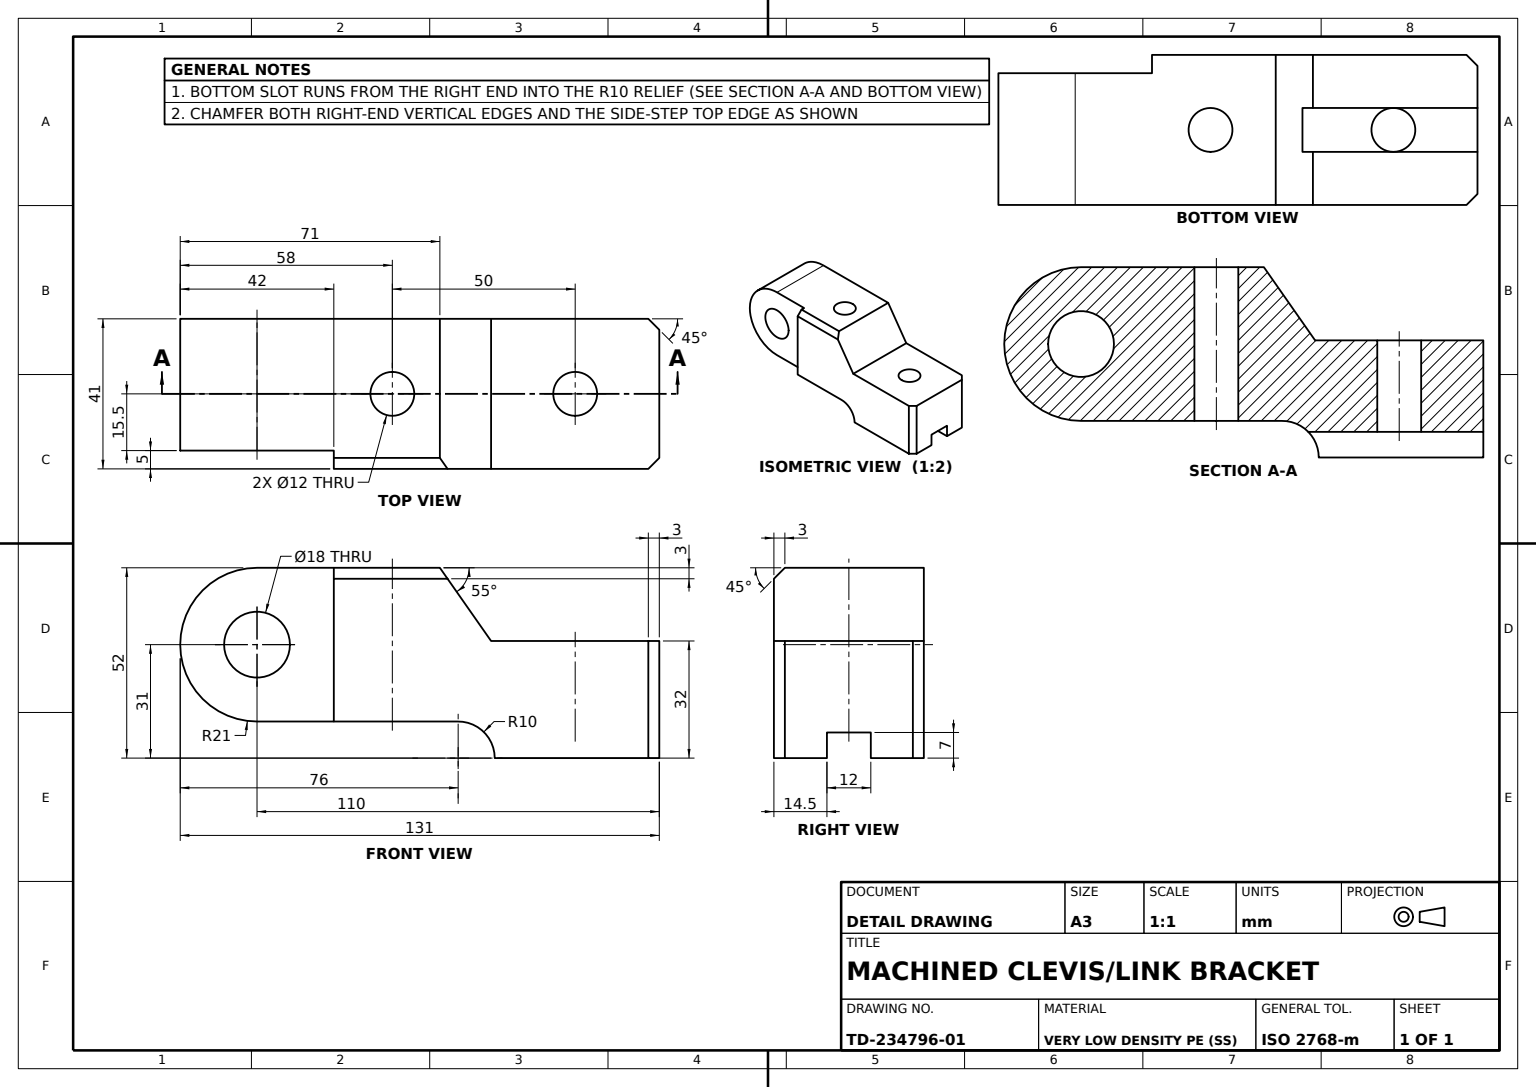
from build123d import *

# Parameters (mm, degrees)
BRACKET_SIDE_PROFILE_SKETCH_R = 9
BRACKET_BODY_41MM_DEPTH       = 20.5
TOP_FACE_CUTS_SKETCH_R        = 6
TOP_FACE_CUTS_SKETCH_W        = 42
TOP_FACE_CUTS_SKETCH_H        = 5
TOP_FACE_CUTS_DEPTH           = 143.425779095
END_SLOT_SKETCH_W             = 12
END_SLOT_SKETCH_H             = 7
END_SLOT_12MM_DEPTH           = 143.425779095
EDGE_CHAMFER_3MM_SIZE         = 3


with BuildPart() as part:
    # Bracket Side Profile Sketch → Bracket Body 41mm (new, symmetric)
    with BuildSketch(Plane.XY):
        with BuildLine():
            Line((0, 0), (-45, 0))
            ThreePointArc((-45, 0), (-47.988718556, 7.130352903), (-55.168386504, 9.998582199))
            Line((-55.168386504, 9.998582199), (-86.000956968, 9.998582199))
            Line((-86.000956968, 9.998582199), (-110, 9.998582199))
            ThreePointArc((-110, 9.998582199), (-131, 30.998582199), (-110, 51.998582199))
            Line((-110, 51.998582199), (-85.996841991, 51.998582199))
            Line((-85.996841991, 51.998582199), (-60, 51.998582199))
            Line((-60, 51.998582199), (-45.996841991, 32))
            Line((-45.996841991, 32), (0, 32))
            Line((0, 32), (0, 0))
        make_face()
        with Locations((-110, 30.998582199)):
            Circle(BRACKET_SIDE_PROFILE_SKETCH_R, mode=Mode.SUBTRACT)
    extrude(amount=BRACKET_BODY_41MM_DEPTH, both=True)

    # Top Face Cuts Sketch → Top Face Cuts (cut, through all)
    with BuildSketch(Plane(origin=(0, 51.998582199, 0), x_dir=(1, 0, 0), z_dir=(0, 1, 0))):
        with Locations(Location((-72.998420995, 0, 0), (0, 0, 270))):
            Circle(TOP_FACE_CUTS_SKETCH_R)
        with Locations(Location((-22.998420995, 0, 0), (0, 0, 270))):
            Circle(TOP_FACE_CUTS_SKETCH_R)
        with Locations((-110, -18)):
            Rectangle(TOP_FACE_CUTS_SKETCH_W, TOP_FACE_CUTS_SKETCH_H)
    extrude(amount=-TOP_FACE_CUTS_DEPTH, mode=Mode.SUBTRACT)

    # End Slot Sketch → End Slot 12mm (cut, through all)
    with BuildSketch(Plane(origin=(0, 0, 0), x_dir=(0, 0, -1), z_dir=(1, 0, 0))):
        with Locations((0, 3.5)):
            Rectangle(END_SLOT_SKETCH_W, END_SLOT_SKETCH_H)
    extrude(amount=-END_SLOT_12MM_DEPTH, mode=Mode.SUBTRACT)

    # Edge Chamfer 3mm
    edge_chamfer_3mm_edges = [part.edges().sort_by_distance(p)[0] for p in [
        (0, 16, -20.5),
        (-74.5, 51.998582199, 20.5),
        (0, 16, 20.5),
    ]]
    chamfer(edge_chamfer_3mm_edges, length=EDGE_CHAMFER_3MM_SIZE)


solid = part.part
